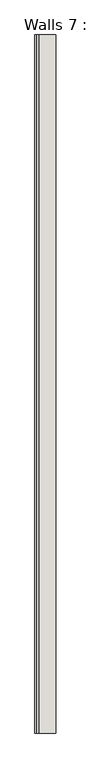
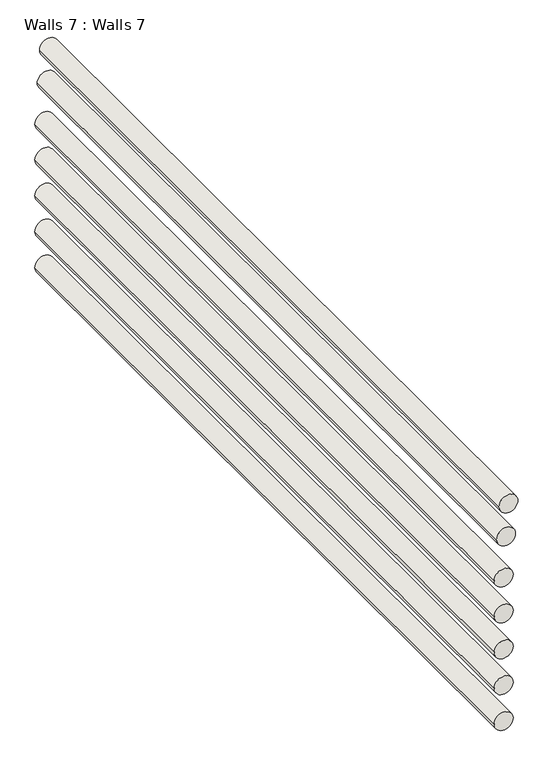
"""IFC4 building model written with IfcOpenShell, lengths in millimetres: wall geometry, Walls 7 : Walls 7."""

from ifc_helpers import new_model, si_unit, point, frame, frame_2d, origin, place, context, project, spatial, circle_curve, trimmed, segment, composite_curve, outline, extrude, source, transform, mapped, element, save


def walls_7_walls_7_87e04c6a(model_context):
    return source(origin(), model_context, "Body", "SweptSolid", [
        extrude(outline(composite_curve([segment(trimmed(circle_curve(frame_2d((4800.1306891, 2094.6271302)), 25.4), [point((4800.1306891, 2120.0271302))], [point((4800.1306891, 2069.2271302))], False, "CARTESIAN"), True, "CONTINUOUS"), segment(trimmed(circle_curve(frame_2d((4800.1306891, 2094.6271302)), 25.4), [point((4800.1306891, 2069.2271302))], [point((4800.1306891, 2120.0271302))], False, "CARTESIAN"), True, "CONTINUOUS")], self_intersect=False)), frame((0.0, 3766.5740351, 0.0), z_axis=(0.0, 1.0, 0.0), x_axis=(0.0, 0.0, 1.0)), (0.0, 0.0, 1.0), 2133.6),
        extrude(outline(composite_curve([segment(trimmed(circle_curve(frame_2d((4709.3075845, 2088.2771302)), 25.4), [point((4709.3075845, 2113.6771302))], [point((4709.3075845, 2062.8771302))], False, "CARTESIAN"), True, "CONTINUOUS"), segment(trimmed(circle_curve(frame_2d((4709.3075845, 2088.2771302)), 25.4), [point((4709.3075845, 2062.8771302))], [point((4709.3075845, 2113.6771302))], False, "CARTESIAN"), True, "CONTINUOUS")], self_intersect=False)), frame((0.0, 3766.5740351, 0.0), z_axis=(0.0, 1.0, 0.0), x_axis=(0.0, 0.0, 1.0)), (0.0, 0.0, 1.0), 2133.6),
        extrude(outline(composite_curve([segment(trimmed(circle_curve(frame_2d((4595.0075845, 2081.9271302)), 25.4), [point((4595.0075845, 2107.3271302))], [point((4595.0075845, 2056.5271302))], False, "CARTESIAN"), True, "CONTINUOUS"), segment(trimmed(circle_curve(frame_2d((4595.0075845, 2081.9271302)), 25.4), [point((4595.0075845, 2056.5271302))], [point((4595.0075845, 2107.3271302))], False, "CARTESIAN"), True, "CONTINUOUS")], self_intersect=False)), frame((0.0, 3766.5740351, 0.0), z_axis=(0.0, 1.0, 0.0), x_axis=(0.0, 0.0, 1.0)), (0.0, 0.0, 1.0), 2133.6),
        extrude(outline(composite_curve([segment(trimmed(circle_curve(frame_2d((4493.4075845, 2081.9271302)), 25.4), [point((4493.4075845, 2107.3271302))], [point((4493.4075845, 2056.5271302))], False, "CARTESIAN"), True, "CONTINUOUS"), segment(trimmed(circle_curve(frame_2d((4493.4075845, 2081.9271302)), 25.4), [point((4493.4075845, 2056.5271302))], [point((4493.4075845, 2107.3271302))], False, "CARTESIAN"), True, "CONTINUOUS")], self_intersect=False)), frame((0.0, 3766.5740351, 0.0), z_axis=(0.0, 1.0, 0.0), x_axis=(0.0, 0.0, 1.0)), (0.0, 0.0, 1.0), 2133.6),
        extrude(outline(composite_curve([segment(trimmed(circle_curve(frame_2d((4391.8075845, 2081.9271302)), 25.4), [point((4391.8075845, 2107.3271302))], [point((4391.8075845, 2056.5271302))], False, "CARTESIAN"), True, "CONTINUOUS"), segment(trimmed(circle_curve(frame_2d((4391.8075845, 2081.9271302)), 25.4), [point((4391.8075845, 2056.5271302))], [point((4391.8075845, 2107.3271302))], False, "CARTESIAN"), True, "CONTINUOUS")], self_intersect=False)), frame((0.0, 3766.5740351, 0.0), z_axis=(0.0, 1.0, 0.0), x_axis=(0.0, 0.0, 1.0)), (0.0, 0.0, 1.0), 2133.6),
        extrude(outline(composite_curve([segment(trimmed(circle_curve(frame_2d((4290.2075845, 2081.9271302)), 25.4), [point((4290.2075845, 2107.3271302))], [point((4290.2075845, 2056.5271302))], False, "CARTESIAN"), True, "CONTINUOUS"), segment(trimmed(circle_curve(frame_2d((4290.2075845, 2081.9271302)), 25.4), [point((4290.2075845, 2056.5271302))], [point((4290.2075845, 2107.3271302))], False, "CARTESIAN"), True, "CONTINUOUS")], self_intersect=False)), frame((0.0, 3766.5740351, 0.0), z_axis=(0.0, 1.0, 0.0), x_axis=(0.0, 0.0, 1.0)), (0.0, 0.0, 1.0), 2133.6),
        extrude(outline(composite_curve([segment(trimmed(circle_curve(frame_2d((4188.6075845, 2081.9271302)), 25.4), [point((4188.6075845, 2107.3271302))], [point((4188.6075845, 2056.5271302))], False, "CARTESIAN"), True, "CONTINUOUS"), segment(trimmed(circle_curve(frame_2d((4188.6075845, 2081.9271302)), 25.4), [point((4188.6075845, 2056.5271302))], [point((4188.6075845, 2107.3271302))], False, "CARTESIAN"), True, "CONTINUOUS")], self_intersect=False)), frame((0.0, 3766.5740351, 0.0), z_axis=(0.0, 1.0, 0.0), x_axis=(0.0, 0.0, 1.0)), (0.0, 0.0, 1.0), 2133.6),
    ])


if __name__ == "__main__":
    model = new_model("IFC4")
    model_context = context("Model", 3, world=origin())
    ifc_project = project(units=[si_unit("LENGTHUNIT", "METRE", prefix="MILLI")], contexts=[model_context])
    site = spatial("IfcSite", under=ifc_project)
    building = spatial("IfcBuilding", under=site)
    placement = place(None, origin())
    walls_7_walls_7_shape = walls_7_walls_7_87e04c6a(model_context)
    element("IfcWall", 1, ObjectType="Walls 7 : Walls 7", at=placement, inside=building, context=model_context, shape_type="MappedRepresentation", body=[
        mapped(walls_7_walls_7_shape, transform((0.0, 0.0, 0.0), x_axis=(1.0, 0.0, 0.0), y_axis=(0.0, 1.0, 0.0), z_axis=(0.0, 0.0, 1.0))),
    ])
    save(model, "model.ifc")

# Revit data of these elements
# Element 1 (IfcWall, "Walls 7 : Walls 7")
#   Materials on its faces: "Default Wall"
# Materials
#   "Default Wall": colour RGB 128 128 128, transparency 0
